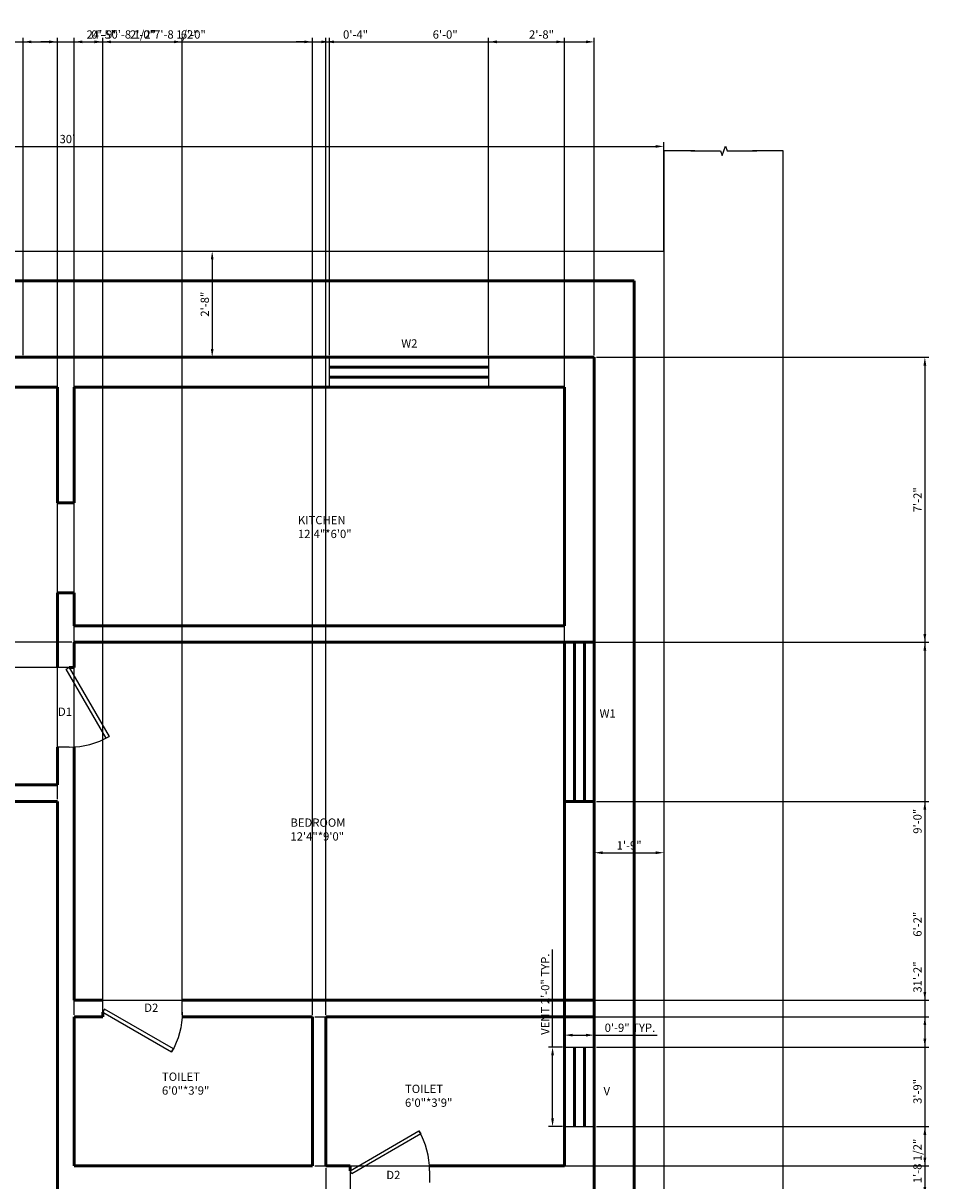
# Model space of a CAD drawing. Units: inches. Extents: x 2020 to 7901, y 1581 to 3943.
# Tile 5 of 17: x 2526 to 2800, y 1966 to 2315. Entities that reach past the tile are written whole.
import ezdxf

# ---------------------------------------------------------------- set-up
doc = ezdxf.new("R2010")
doc.units = ezdxf.units.IN
for name, color, linetype, lineweight in [('A-ANNO-DIMS', 2, 'Continuous', 18), ('A-ANNO-TEXT', 7, 'Continuous', 18), ('A-AREA-IDEN', 3, 'Continuous', 18), ('A-DOOR', 4, 'Continuous', 25), ('A-GLAZ', 4, 'Continuous', 25), ('A-WALL', 7, 'Continuous', 50), ('C-PROP', 6, 'Continuous', 25)]:
    doc.layers.add(name, color=color, linetype=linetype, lineweight=lineweight)
doc.styles.get("Standard").update_dxf_attribs({"font": 'arial.ttf'})
doc.dimstyles.new('ISO-25', dxfattribs={"dimtxt": 2.5, "dimasz": 2.5, "dimexe": 1.25, "dimexo": 0.625, "dimtad": 1, "dimdec": 1, "dimlunit": 3, "dimtxsty": 'Standard', "dimcen": 2.5, "dimadec": 0, "dimazin": 0, "dimtfac": 1, "dimtdec": 1, "dimtmove": 0, "dimatfit": 3, "dimfxl": 1, "dimarcsym": 0})

# ---------------------------------------------------------------- blocks, each defined once
blk = doc.blocks.new('*U2')
for p, q in [((0, 0), (0, -6)), ((40, 0), (40, -6))]:
    blk.add_line(p, q)
blk.add_lwpolyline([(0, 0), (34.64, 20), (35.52, 18.48), (0.87, -1.52)], close=True)
blk.add_arc((0, 0), 40, 0, 30)
blk = doc.blocks.new('*D6')
at = {"layer": 'A-ANNO-DIMS', "color": 0, "lineweight": -2, "transparency": 16777216}
for p, q in [((2574.55, 2246.34), (2583.91, 2246.34)), ((2582.66, 2243.84), (2582.66, 2216.84)), ((2574.55, 2214.34), (2583.91, 2214.34))]:
    blk.add_line(p, q, dxfattribs=at)
at = {"layer": 'A-ANNO-DIMS', "color": 0, "transparency": 16777216}
for points in [[(2582.24, 2243.84), (2583.08, 2243.84), (2582.66, 2246.34)], [(2582.24, 2216.84), (2583.08, 2216.84), (2582.66, 2214.34)]]:
    blk.add_solid(points, dxfattribs=at)
at = {"layer": 'DEFPOINTS', "color": 0, "transparency": 16777216}
for p in [(2573.92, 2246.34), (2573.92, 2214.34), (2582.66, 2214.34)]:
    blk.add_point(p, dxfattribs=at)
at = {"layer": 'A-ANNO-DIMS', "color": 0, "transparency": 16777216, "insert": (2580.76, 2230.34), "char_height": 2.5, "attachment_point": 5, "rotation": 90}
blk.add_mtext('2\'-8"', dxfattribs=at)
blk = doc.blocks.new('*D7')
at = {"layer": 'A-ANNO-DIMS', "color": 0, "lineweight": -2, "transparency": 16777216}
for p, q in [((2697.96, 2068.17), (2697.96, 2063.6)), ((2718.96, 2068.17), (2718.96, 2063.6)), ((2700.46, 2064.85), (2716.46, 2064.85))]:
    blk.add_line(p, q, dxfattribs=at)
at = {"layer": 'A-ANNO-DIMS', "color": 0, "transparency": 16777216}
for points in [[(2700.46, 2065.27), (2700.46, 2064.43), (2697.96, 2064.85)], [(2716.46, 2065.27), (2716.46, 2064.43), (2718.96, 2064.85)]]:
    blk.add_solid(points, dxfattribs=at)
at = {"layer": 'DEFPOINTS', "color": 0, "transparency": 16777216}
for p in [(2697.96, 2068.8), (2718.96, 2068.8), (2718.96, 2064.85)]:
    blk.add_point(p, dxfattribs=at)
at = {"layer": 'A-ANNO-DIMS', "color": 0, "transparency": 16777216, "insert": (2708.46, 2066.75), "char_height": 2.5, "attachment_point": 5}
blk.add_mtext('1\'-9"', dxfattribs=at)
blk = doc.blocks.new('*D8')
at = {"layer": 'A-ANNO-DIMS', "color": 0, "lineweight": -2, "transparency": 16777216}
for p, q in [((2358.96, 2246.96), (2358.96, 2279.19)), ((2361.46, 2277.94), (2716.46, 2277.94)), ((2718.96, 2246.96), (2718.96, 2279.19))]:
    blk.add_line(p, q, dxfattribs=at)
at = {"layer": 'A-ANNO-DIMS', "color": 0, "transparency": 16777216}
for points in [[(2361.46, 2278.35), (2361.46, 2277.52), (2358.96, 2277.94)], [(2716.46, 2278.35), (2716.46, 2277.52), (2718.96, 2277.94)]]:
    blk.add_solid(points, dxfattribs=at)
at = {"layer": 'DEFPOINTS', "color": 0, "transparency": 16777216}
for p in [(2718.96, 2277.94), (2358.96, 2246.34), (2718.96, 2246.34)]:
    blk.add_point(p, dxfattribs=at)
at = {"layer": 'A-ANNO-DIMS', "color": 0, "transparency": 16777216, "insert": (2538.96, 2279.84), "char_height": 2.5, "attachment_point": 5}
blk.add_mtext("30'", dxfattribs=at)
blk = doc.blocks.new('WIN-1200')
for p, q in [((0, 9), (48, 9)), ((0, 0), (0, 9)), ((48, 9), (48, 0)), ((48, 0), (0, 0))]:
    blk.add_line(p, q)
blk = doc.blocks.new('VENT-600')
for p, q in [((0, 24), (9, 24)), ((0, 24), (0, 0)), ((9, 0), (9, 24)), ((0, 0), (9, 0))]:
    blk.add_line(p, q)
blk = doc.blocks.new('*D27')
at = {"layer": 'A-ANNO-DIMS', "color": 0, "lineweight": -2, "transparency": 16777216}
for p, q in [((2685.36, 2006.22), (2685.36, 2035.62)), ((2688.34, 2006.22), (2684.11, 2006.22)), ((2685.36, 1984.72), (2685.36, 2003.72)), ((2688.34, 1982.22), (2684.11, 1982.22))]:
    blk.add_line(p, q, dxfattribs=at)
at = {"layer": 'A-ANNO-DIMS', "color": 0, "transparency": 16777216}
for points in [[(2684.95, 2003.72), (2685.78, 2003.72), (2685.36, 2006.22)], [(2684.95, 1984.72), (2685.78, 1984.72), (2685.36, 1982.22)]]:
    blk.add_solid(points, dxfattribs=at)
at = {"layer": 'DEFPOINTS', "color": 0, "transparency": 16777216}
for p in [(2685.36, 2006.22), (2688.96, 2006.22), (2688.96, 1982.22)]:
    blk.add_point(p, dxfattribs=at)
at = {"layer": 'A-ANNO-DIMS', "color": 0, "transparency": 16777216, "insert": (2683.46, 2022.17), "char_height": 2.5, "attachment_point": 5, "rotation": 90}
blk.add_mtext('VENT 2\'-0" TYP.', dxfattribs=at)
blk = doc.blocks.new('*D28')
at = {"layer": 'A-ANNO-DIMS', "color": 0, "lineweight": -2, "transparency": 16777216}
for p, q in [((2688.96, 2006.84), (2688.96, 2011.07)), ((2691.46, 2009.82), (2695.46, 2009.82)), ((2697.96, 2006.84), (2697.96, 2011.07)), ((2697.96, 2009.82), (2716.95, 2009.82))]:
    blk.add_line(p, q, dxfattribs=at)
at = {"layer": 'A-ANNO-DIMS', "color": 0, "transparency": 16777216}
for points in [[(2691.46, 2010.23), (2691.46, 2009.4), (2688.96, 2009.82)], [(2695.46, 2010.23), (2695.46, 2009.4), (2697.96, 2009.82)]]:
    blk.add_solid(points, dxfattribs=at)
at = {"layer": 'DEFPOINTS', "color": 0, "transparency": 16777216}
for p in [(2697.96, 2009.82), (2688.96, 2006.22), (2697.96, 2006.22)]:
    blk.add_point(p, dxfattribs=at)
at = {"layer": 'A-ANNO-DIMS', "color": 0, "transparency": 16777216, "insert": (2708.71, 2011.72), "char_height": 2.5, "attachment_point": 5}
blk.add_mtext('0\'-9" TYP.', dxfattribs=at)
blk = doc.blocks.new('*D32')
at = {"layer": 'A-ANNO-DIMS', "color": 0, "lineweight": -2, "transparency": 16777216}
for p, q in [((2525.61, 2214.96), (2525.61, 2310.73)), ((2528.11, 2309.48), (2615.57, 2309.48)), ((2618.07, 2214.96), (2618.07, 2310.73))]:
    blk.add_line(p, q, dxfattribs=at)
at = {"layer": 'A-ANNO-DIMS', "color": 0, "transparency": 16777216}
for points in [[(2528.11, 2309.9), (2528.11, 2309.07), (2525.61, 2309.48)], [(2615.57, 2309.9), (2615.57, 2309.07), (2618.07, 2309.48)]]:
    blk.add_solid(points, dxfattribs=at)
at = {"layer": 'DEFPOINTS', "color": 0, "transparency": 16777216}
for p in [(2618.07, 2309.48), (2525.61, 2214.34), (2618.07, 2214.34)]:
    blk.add_point(p, dxfattribs=at)
at = {"layer": 'A-ANNO-DIMS', "color": 0, "transparency": 16777216, "insert": (2571.84, 2311.4), "char_height": 2.5, "attachment_point": 5}
blk.add_mtext('7\'-8 1/2"', dxfattribs=at)
blk = doc.blocks.new('*D33')
at = {"layer": 'A-ANNO-DIMS', "color": 0, "lineweight": -2, "transparency": 16777216}
for p, q in [((2666.07, 2214.96), (2666.07, 2310.73)), ((2668.57, 2309.48), (2695.46, 2309.48)), ((2697.96, 2214.96), (2697.96, 2310.73))]:
    blk.add_line(p, q, dxfattribs=at)
at = {"layer": 'A-ANNO-DIMS', "color": 0, "transparency": 16777216}
for points in [[(2668.57, 2309.9), (2668.57, 2309.07), (2666.07, 2309.48)], [(2695.46, 2309.9), (2695.46, 2309.07), (2697.96, 2309.48)]]:
    blk.add_solid(points, dxfattribs=at)
at = {"layer": 'DEFPOINTS', "color": 0, "transparency": 16777216}
for p in [(2697.96, 2309.48), (2666.07, 2214.34), (2697.96, 2214.34)]:
    blk.add_point(p, dxfattribs=at)
at = {"layer": 'A-ANNO-DIMS', "color": 0, "transparency": 16777216, "insert": (2682.02, 2311.38), "char_height": 2.5, "attachment_point": 5}
blk.add_mtext('2\'-8"', dxfattribs=at)
blk = doc.blocks.new('*D34')
at = {"layer": 'A-ANNO-DIMS', "color": 0, "lineweight": -2, "transparency": 16777216}
for p, q in [((2698.59, 2214.34), (2798.95, 2214.34)), ((2797.7, 2211.84), (2797.7, 2130.84)), ((2698.59, 2128.34), (2798.95, 2128.34))]:
    blk.add_line(p, q, dxfattribs=at)
at = {"layer": 'A-ANNO-DIMS', "color": 0, "transparency": 16777216}
for points in [[(2797.28, 2211.84), (2798.12, 2211.84), (2797.7, 2214.34)], [(2797.28, 2130.84), (2798.12, 2130.84), (2797.7, 2128.34)]]:
    blk.add_solid(points, dxfattribs=at)
at = {"layer": 'DEFPOINTS', "color": 0, "transparency": 16777216}
for p in [(2697.96, 2214.34), (2697.96, 2128.34), (2797.7, 2128.34)]:
    blk.add_point(p, dxfattribs=at)
at = {"layer": 'A-ANNO-DIMS', "color": 0, "transparency": 16777216, "insert": (2795.82, 2171.34), "char_height": 2.5, "attachment_point": 5, "rotation": 90}
blk.add_mtext('7\'-2"', dxfattribs=at)
blk = doc.blocks.new('*D35')
at = {"layer": 'A-ANNO-DIMS', "color": 0, "lineweight": -2, "transparency": 16777216}
for p, q in [((2698.59, 2080.34), (2798.95, 2080.34)), ((2797.7, 2077.84), (2797.7, 2008.72)), ((2698.59, 2006.22), (2798.95, 2006.22))]:
    blk.add_line(p, q, dxfattribs=at)
at = {"layer": 'A-ANNO-DIMS', "color": 0, "transparency": 16777216}
for points in [[(2797.28, 2077.84), (2798.12, 2077.84), (2797.7, 2080.34)], [(2797.28, 2008.72), (2798.12, 2008.72), (2797.7, 2006.22)]]:
    blk.add_solid(points, dxfattribs=at)
at = {"layer": 'DEFPOINTS', "color": 0, "transparency": 16777216}
for p in [(2697.96, 2080.34), (2697.96, 2006.22), (2797.7, 2006.22)]:
    blk.add_point(p, dxfattribs=at)
at = {"layer": 'A-ANNO-DIMS', "color": 0, "transparency": 16777216, "insert": (2795.8, 2043.28), "char_height": 2.5, "attachment_point": 5, "rotation": 90}
blk.add_mtext('6\'-2"', dxfattribs=at)
blk = doc.blocks.new('*D36')
at = {"layer": 'A-ANNO-DIMS', "color": 0, "lineweight": -2, "transparency": 16777216}
for p, q in [((2698.59, 1982.22), (2798.95, 1982.22)), ((2797.7, 1979.72), (2797.7, 1964)), ((2698.59, 1961.5), (2798.95, 1961.5))]:
    blk.add_line(p, q, dxfattribs=at)
at = {"layer": 'A-ANNO-DIMS', "color": 0, "transparency": 16777216}
for points in [[(2797.28, 1979.72), (2798.12, 1979.72), (2797.7, 1982.22)], [(2797.28, 1964), (2798.12, 1964), (2797.7, 1961.5)]]:
    blk.add_solid(points, dxfattribs=at)
at = {"layer": 'DEFPOINTS', "color": 0, "transparency": 16777216}
for p in [(2697.96, 1982.22), (2697.96, 1961.5), (2797.7, 1961.5)]:
    blk.add_point(p, dxfattribs=at)
at = {"layer": 'A-ANNO-DIMS', "color": 0, "transparency": 16777216, "insert": (2795.78, 1971.86), "char_height": 2.5, "attachment_point": 5, "rotation": 90}
blk.add_mtext('1\'-8 1/2"', dxfattribs=at)
blk = doc.blocks.new('*D95')
at = {"layer": 'A-ANNO-DIMS', "color": 0, "lineweight": -2, "transparency": 16777216}
for p, q in [((2400.96, 2214.96), (2400.96, 2310.73)), ((2403.46, 2309.48), (2695.46, 2309.48)), ((2697.96, 2214.96), (2697.96, 2310.73))]:
    blk.add_line(p, q, dxfattribs=at)
at = {"layer": 'A-ANNO-DIMS', "color": 0, "transparency": 16777216}
for points in [[(2403.46, 2309.9), (2403.46, 2309.07), (2400.96, 2309.48)], [(2695.46, 2309.9), (2695.46, 2309.07), (2697.96, 2309.48)]]:
    blk.add_solid(points, dxfattribs=at)
at = {"layer": 'DEFPOINTS', "color": 0, "transparency": 16777216}
for p in [(2697.96, 2309.48), (2400.96, 2214.34), (2697.96, 2214.34)]:
    blk.add_point(p, dxfattribs=at)
at = {"layer": 'A-ANNO-DIMS', "color": 0, "transparency": 16777216, "insert": (2549.46, 2311.38), "char_height": 2.5, "attachment_point": 5}
blk.add_mtext('24\'-9"', dxfattribs=at)
blk = doc.blocks.new('*D96')
at = {"layer": 'A-ANNO-DIMS', "color": 0, "lineweight": -2, "transparency": 16777216}
for p, q in [((2698.59, 2214.34), (2798.95, 2214.34)), ((2797.7, 2211.84), (2797.7, 1842.84)), ((2698.59, 1840.34), (2798.95, 1840.34))]:
    blk.add_line(p, q, dxfattribs=at)
at = {"layer": 'A-ANNO-DIMS', "color": 0, "transparency": 16777216}
for points in [[(2797.28, 2211.84), (2798.12, 2211.84), (2797.7, 2214.34)], [(2797.28, 1842.84), (2798.12, 1842.84), (2797.7, 1840.34)]]:
    blk.add_solid(points, dxfattribs=at)
at = {"layer": 'DEFPOINTS', "color": 0, "transparency": 16777216}
for p in [(2697.96, 2214.34), (2697.96, 1840.34), (2797.7, 1840.34)]:
    blk.add_point(p, dxfattribs=at)
at = {"layer": 'A-ANNO-DIMS', "color": 0, "transparency": 16777216, "insert": (2795.8, 2027.34), "char_height": 2.5, "attachment_point": 5, "rotation": 90}
blk.add_mtext('31\'-2"', dxfattribs=at)
blk = doc.blocks.new('*D99')
at = {"layer": 'A-ANNO-DIMS', "color": 0, "lineweight": -2, "transparency": 16777216}
for p, q in [((2541.59, 2128.34), (2798.95, 2128.34)), ((2797.7, 2125.84), (2797.7, 2022.84)), ((2541.59, 2020.34), (2798.95, 2020.34))]:
    blk.add_line(p, q, dxfattribs=at)
at = {"layer": 'A-ANNO-DIMS', "color": 0, "transparency": 16777216}
for points in [[(2797.28, 2125.84), (2798.12, 2125.84), (2797.7, 2128.34)], [(2797.28, 2022.84), (2798.12, 2022.84), (2797.7, 2020.34)]]:
    blk.add_solid(points, dxfattribs=at)
at = {"layer": 'DEFPOINTS', "color": 0, "transparency": 16777216}
for p in [(2540.96, 2128.34), (2540.96, 2020.34), (2797.7, 2020.34)]:
    blk.add_point(p, dxfattribs=at)
at = {"layer": 'A-ANNO-DIMS', "color": 0, "transparency": 16777216, "insert": (2795.8, 2074.34), "char_height": 2.5, "attachment_point": 5, "rotation": 90}
blk.add_mtext('9\'-0"', dxfattribs=at)
blk = doc.blocks.new('*D100')
at = {"layer": 'A-ANNO-DIMS', "color": 0, "lineweight": -2, "transparency": 16777216}
for p, q in [((2613.59, 2015.34), (2798.95, 2015.34)), ((2797.7, 2012.84), (2797.7, 1972.84)), ((2613.59, 1970.34), (2798.95, 1970.34))]:
    blk.add_line(p, q, dxfattribs=at)
at = {"layer": 'A-ANNO-DIMS', "color": 0, "transparency": 16777216}
for points in [[(2797.28, 2012.84), (2798.12, 2012.84), (2797.7, 2015.34)], [(2797.28, 1972.84), (2798.12, 1972.84), (2797.7, 1970.34)]]:
    blk.add_solid(points, dxfattribs=at)
at = {"layer": 'DEFPOINTS', "color": 0, "transparency": 16777216}
for p in [(2612.96, 2015.34), (2612.96, 1970.34), (2797.7, 1970.34)]:
    blk.add_point(p, dxfattribs=at)
at = {"layer": 'A-ANNO-DIMS', "color": 0, "transparency": 16777216, "insert": (2795.8, 1992.84), "char_height": 2.5, "attachment_point": 5, "rotation": 90}
blk.add_mtext('3\'-9"', dxfattribs=at)
blk = doc.blocks.new('*D102')
at = {"layer": 'A-ANNO-DIMS', "color": 0, "lineweight": -2, "transparency": 16777216}
for p, q in [((2533.46, 2309.48), (2530.96, 2309.48)), ((2535.96, 2080.96), (2535.96, 2310.73)), ((2535.96, 2309.48), (2540.96, 2309.48)), ((2540.96, 2097.4), (2540.96, 2310.73)), ((2543.46, 2309.48), (2553.86, 2309.48))]:
    blk.add_line(p, q, dxfattribs=at)
at = {"layer": 'A-ANNO-DIMS', "color": 0, "transparency": 16777216}
for points in [[(2533.46, 2309.9), (2533.46, 2309.07), (2535.96, 2309.48)], [(2543.46, 2309.9), (2543.46, 2309.07), (2540.96, 2309.48)]]:
    blk.add_solid(points, dxfattribs=at)
at = {"layer": 'DEFPOINTS', "color": 0, "transparency": 16777216}
for p in [(2540.96, 2309.48), (2540.96, 2096.78), (2535.96, 2080.34)]:
    blk.add_point(p, dxfattribs=at)
at = {"layer": 'A-ANNO-DIMS', "color": 0, "transparency": 16777216, "insert": (2549.91, 2311.38), "char_height": 2.5, "attachment_point": 5}
blk.add_mtext('0\'-5"', dxfattribs=at)
blk = doc.blocks.new('*D103')
at = {"layer": 'A-ANNO-DIMS', "color": 0, "lineweight": -2, "transparency": 16777216}
for p, q in [((2540.96, 2015.96), (2540.96, 2310.73)), ((2543.46, 2309.48), (2610.46, 2309.48)), ((2612.96, 2015.96), (2612.96, 2310.73))]:
    blk.add_line(p, q, dxfattribs=at)
at = {"layer": 'A-ANNO-DIMS', "color": 0, "transparency": 16777216}
for points in [[(2543.46, 2309.9), (2543.46, 2309.07), (2540.96, 2309.48)], [(2610.46, 2309.9), (2610.46, 2309.07), (2612.96, 2309.48)]]:
    blk.add_solid(points, dxfattribs=at)
at = {"layer": 'DEFPOINTS', "color": 0, "transparency": 16777216}
for p in [(2612.96, 2309.48), (2540.96, 2015.34), (2612.96, 2015.34)]:
    blk.add_point(p, dxfattribs=at)
at = {"layer": 'A-ANNO-DIMS', "color": 0, "transparency": 16777216, "insert": (2576.96, 2311.38), "char_height": 2.5, "attachment_point": 5}
blk.add_mtext('6\'-0"', dxfattribs=at)
blk = doc.blocks.new('*D104')
at = {"layer": 'A-ANNO-DIMS', "color": 0, "lineweight": -2, "transparency": 16777216}
for p, q in [((2610.46, 2309.48), (2607.96, 2309.48)), ((2612.96, 2015.96), (2612.96, 2310.73)), ((2612.96, 2309.48), (2616.96, 2309.48)), ((2616.96, 2015.96), (2616.96, 2310.73)), ((2619.46, 2309.48), (2629.86, 2309.48))]:
    blk.add_line(p, q, dxfattribs=at)
at = {"layer": 'A-ANNO-DIMS', "color": 0, "transparency": 16777216}
for points in [[(2610.46, 2309.9), (2610.46, 2309.07), (2612.96, 2309.48)], [(2619.46, 2309.9), (2619.46, 2309.07), (2616.96, 2309.48)]]:
    blk.add_solid(points, dxfattribs=at)
at = {"layer": 'DEFPOINTS', "color": 0, "transparency": 16777216}
for p in [(2616.96, 2309.48), (2612.96, 2015.34), (2616.96, 2015.34)]:
    blk.add_point(p, dxfattribs=at)
at = {"layer": 'A-ANNO-DIMS', "color": 0, "transparency": 16777216, "insert": (2625.91, 2311.38), "char_height": 2.5, "attachment_point": 5}
blk.add_mtext('0\'-4"', dxfattribs=at)
blk = doc.blocks.new('*D105')
at = {"layer": 'A-ANNO-DIMS', "color": 0, "lineweight": -2, "transparency": 16777216}
for p, q in [((2616.96, 2015.96), (2616.96, 2310.73)), ((2619.46, 2309.48), (2686.46, 2309.48)), ((2688.96, 2006.84), (2688.96, 2310.73))]:
    blk.add_line(p, q, dxfattribs=at)
at = {"layer": 'A-ANNO-DIMS', "color": 0, "transparency": 16777216}
for points in [[(2619.46, 2309.9), (2619.46, 2309.07), (2616.96, 2309.48)], [(2686.46, 2309.9), (2686.46, 2309.07), (2688.96, 2309.48)]]:
    blk.add_solid(points, dxfattribs=at)
at = {"layer": 'DEFPOINTS', "color": 0, "transparency": 16777216}
for p in [(2688.96, 2309.48), (2616.96, 2015.34), (2688.96, 2006.22)]:
    blk.add_point(p, dxfattribs=at)
at = {"layer": 'A-ANNO-DIMS', "color": 0, "transparency": 16777216, "insert": (2652.96, 2311.38), "char_height": 2.5, "attachment_point": 5}
blk.add_mtext('6\'-0"', dxfattribs=at)
blk = doc.blocks.new('*D107')
at = {"layer": 'A-ANNO-DIMS', "color": 0, "lineweight": -2, "transparency": 16777216}
for p, q in [((2479.8, 2080.96), (2479.8, 2310.73)), ((2482.3, 2309.48), (2533.46, 2309.48)), ((2535.96, 2080.96), (2535.96, 2310.73))]:
    blk.add_line(p, q, dxfattribs=at)
at = {"layer": 'A-ANNO-DIMS', "color": 0, "transparency": 16777216}
for points in [[(2482.3, 2309.9), (2482.3, 2309.07), (2479.8, 2309.48)], [(2533.46, 2309.9), (2533.46, 2309.07), (2535.96, 2309.48)]]:
    blk.add_solid(points, dxfattribs=at)
at = {"layer": 'DEFPOINTS', "color": 0, "transparency": 16777216}
for p in [(2535.96, 2309.48), (2479.8, 2080.34), (2535.96, 2080.34)]:
    blk.add_point(p, dxfattribs=at)
at = {"layer": 'A-ANNO-DIMS', "color": 0, "transparency": 16777216, "insert": (2507.88, 2311.38), "char_height": 2.5, "attachment_point": 5}
blk.add_mtext('4\'-8"', dxfattribs=at)
blk = doc.blocks.new('*D111')
at = {"layer": 'A-ANNO-DIMS', "color": 0, "lineweight": -2, "transparency": 16777216}
for p, q in [((2540.34, 2128.34), (2272.67, 2128.34)), ((2273.92, 2125.84), (2273.92, 2123.23)), ((2540.34, 2120.73), (2272.67, 2120.73)), ((2273.92, 2120.73), (2273.92, 2104.51))]:
    blk.add_line(p, q, dxfattribs=at)
at = {"layer": 'A-ANNO-DIMS', "color": 0, "transparency": 16777216}
for points in [[(2273.5, 2125.84), (2274.33, 2125.84), (2273.92, 2128.34)], [(2273.5, 2123.23), (2274.33, 2123.23), (2273.92, 2120.73)]]:
    blk.add_solid(points, dxfattribs=at)
at = {"layer": 'DEFPOINTS', "color": 0, "transparency": 16777216}
for p in [(2540.96, 2128.34), (2273.92, 2120.73), (2540.96, 2120.73)]:
    blk.add_point(p, dxfattribs=at)
at = {"layer": 'A-ANNO-DIMS', "color": 0, "transparency": 16777216, "insert": (2272, 2111.37), "char_height": 2.5, "attachment_point": 5, "rotation": 90}
blk.add_mtext('0\'-7 1/2"', dxfattribs=at)
blk = doc.blocks.new('*D114')
at = {"layer": 'A-ANNO-DIMS', "color": 0, "lineweight": -2, "transparency": 16777216}
for p, q in [((2540.96, 2020.96), (2540.96, 2310.73)), ((2543.46, 2309.48), (2547.13, 2309.48)), ((2549.63, 2020.96), (2549.63, 2310.73)), ((2549.63, 2309.48), (2565.85, 2309.48))]:
    blk.add_line(p, q, dxfattribs=at)
at = {"layer": 'A-ANNO-DIMS', "color": 0, "transparency": 16777216}
for points in [[(2543.46, 2309.9), (2543.46, 2309.07), (2540.96, 2309.48)], [(2547.13, 2309.9), (2547.13, 2309.07), (2549.63, 2309.48)]]:
    blk.add_solid(points, dxfattribs=at)
at = {"layer": 'DEFPOINTS', "color": 0, "transparency": 16777216}
for p in [(2549.63, 2309.48), (2540.96, 2020.34), (2549.63, 2020.34)]:
    blk.add_point(p, dxfattribs=at)
at = {"layer": 'A-ANNO-DIMS', "color": 0, "transparency": 16777216, "insert": (2558.99, 2311.4), "char_height": 2.5, "attachment_point": 5}
blk.add_mtext('0\'-8 1/2"', dxfattribs=at)
blk = doc.blocks.new('*D115')
at = {"layer": 'A-ANNO-DIMS', "color": 0, "lineweight": -2, "transparency": 16777216}
for p, q in [((2549.63, 2015.96), (2549.63, 2310.73)), ((2552.13, 2309.48), (2571.09, 2309.48)), ((2573.59, 2015.96), (2573.59, 2310.73))]:
    blk.add_line(p, q, dxfattribs=at)
at = {"layer": 'A-ANNO-DIMS', "color": 0, "transparency": 16777216}
for points in [[(2552.13, 2309.9), (2552.13, 2309.07), (2549.63, 2309.48)], [(2571.09, 2309.9), (2571.09, 2309.07), (2573.59, 2309.48)]]:
    blk.add_solid(points, dxfattribs=at)
at = {"layer": 'DEFPOINTS', "color": 0, "transparency": 16777216}
for p in [(2573.59, 2309.48), (2549.63, 2015.34), (2573.59, 2015.34)]:
    blk.add_point(p, dxfattribs=at)
at = {"layer": 'A-ANNO-DIMS', "color": 0, "transparency": 16777216, "insert": (2561.61, 2311.38), "char_height": 2.5, "attachment_point": 5}
blk.add_mtext('2\'-0"', dxfattribs=at)
blk = doc.blocks.new('*D116')
at = {"layer": 'A-ANNO-DIMS', "color": 0, "lineweight": -2, "transparency": 16777216}
for p, q in [((2616.96, 1969.71), (2616.96, 1664.26)), ((2624.26, 1969.71), (2624.26, 1664.26)), ((2619.46, 1665.51), (2621.76, 1665.51)), ((2624.26, 1665.51), (2640.48, 1665.51))]:
    blk.add_line(p, q, dxfattribs=at)
at = {"layer": 'A-ANNO-DIMS', "color": 0, "transparency": 16777216}
for points in [[(2619.46, 1665.92), (2619.46, 1665.09), (2616.96, 1665.51)], [(2621.76, 1665.92), (2621.76, 1665.09), (2624.26, 1665.51)]]:
    blk.add_solid(points, dxfattribs=at)
at = {"layer": 'DEFPOINTS', "color": 0, "transparency": 16777216}
for p in [(2616.96, 1970.34), (2624.26, 1970.34), (2624.26, 1665.51)]:
    blk.add_point(p, dxfattribs=at)
at = {"layer": 'A-ANNO-DIMS', "color": 0, "transparency": 16777216, "insert": (2633.62, 1667.43), "char_height": 2.5, "attachment_point": 5}
blk.add_mtext('0\'-7 1/2"', dxfattribs=at)

msp = doc.modelspace()

# ---------------------------------------------------------------- linework, layer by layer
at = {"layer": 'A-WALL'}
for p, q in [((2367.96, 2237.34), (2709.96, 2237.34)), ((2709.96, 2237.34), (2709.96, 1766.34)), ((2446.34, 2214.34), (2697.96, 2214.34)), ((2618.07, 2211.34), (2666.07, 2211.34)), ((2697.96, 2214.34), (2697.96, 1766.34)), ((2666.07, 2208.34), (2618.07, 2208.34)), ((2446.34, 2205.34), (2535.96, 2205.34)), ((2535.96, 2170.42), (2535.96, 2205.34)), ((2540.96, 2205.34), (2540.96, 2170.42)), ((2540.96, 2205.34), (2688.96, 2205.34)), ((2688.96, 2205.34), (2688.96, 2133.34)), ((2535.96, 2170.42), (2540.96, 2170.42)), ((2535.96, 2143.26), (2540.96, 2143.26)), ((2535.96, 2120.73), (2535.96, 2143.26)), ((2540.96, 2143.26), (2540.96, 2133.34)), ((2540.96, 2133.34), (2688.96, 2133.34)), ((2540.96, 2128.34), (2697.96, 2128.34)), ((2540.96, 2128.34), (2540.96, 2120.73)), ((2688.96, 2080.34), (2688.96, 2128.34)), ((2688.96, 2128.34), (2697.96, 2128.34)), ((2688.96, 2128.34), (2688.96, 1970.34)), ((2691.96, 2080.34), (2691.96, 2128.34)), ((2694.96, 2128.34), (2694.96, 2080.34)), ((2697.96, 2128.34), (2697.96, 2080.34)), ((2539.55, 2120.73), (2540.96, 2120.73)), ((2535.96, 2085.34), (2535.96, 2096.73)), ((2540.96, 2096.78), (2540.96, 2020.34)), ((2479.8, 2085.34), (2535.96, 2085.34)), ((2479.8, 2080.34), (2535.96, 2080.34)), ((2535.96, 1956.67), (2535.96, 2080.34)), ((2697.96, 2080.34), (2688.96, 2080.34)), ((2540.96, 2020.34), (2549.63, 2020.34)), ((2573.63, 2020.34), (2697.96, 2020.34)), ((2540.96, 2015.34), (2549.63, 2015.34)), ((2540.96, 2015.34), (2540.96, 1970.34)), ((2549.63, 2016.74), (2549.63, 2015.34)), ((2573.59, 2015.34), (2612.96, 2015.34)), ((2612.96, 2015.34), (2612.96, 1970.34)), ((2616.96, 2015.34), (2616.96, 1970.34)), ((2616.96, 2015.34), (2697.96, 2015.34)), ((2691.96, 2006.22), (2691.96, 1982.22)), ((2694.96, 1982.22), (2694.96, 2006.22)), ((2540.96, 1970.34), (2612.96, 1970.34)), ((2616.96, 1970.34), (2624.26, 1970.34)), ((2624.26, 1968.92), (2624.26, 1970.34)), ((2648.22, 1970.34), (2688.96, 1970.34))]:
    msp.add_line(p, q, dxfattribs=at)
at = {"layer": 'C-PROP'}
for p, q in [((2718.96, 2276.61), (2718.96, 2246.34)), ((2728.34, 2276.61), (2718.96, 2276.61)), ((2718.96, 2246.34), (2718.96, 2276.61)), ((2718.96, 2246.34), (2718.96, 2276.61)), ((2754.96, 2276.61), (2745.74, 2276.61)), ((2754.96, 1766.34), (2754.96, 2276.61)), ((2358.96, 2246.34), (2718.96, 2246.34)), ((2718.96, 2246.34), (2718.96, 1766.34))]:
    msp.add_line(p, q, dxfattribs=at)
msp.add_lwpolyline([(2727.09, 2276.61), (2736.04, 2276.61), (2736.54, 2275.24), (2737.54, 2277.98), (2738.04, 2276.61), (2746.99, 2276.61)], dxfattribs=at)

# ---------------------------------------------------------------- block references
at = {"layer": 'A-DOOR', "yscale": 0.6, "zscale": 0.6}
for p, xscale, rotation in [((2539.55, 2120.73), 0.6, 270), ((2549.63, 2016.74), -0.6, 180)]:
    msp.add_blockref('*U2', p, dxfattribs=dict(at, xscale=xscale, rotation=rotation))
at = {"layer": 'A-DOOR', "xscale": 0.6, "yscale": 0.6, "zscale": 0.6}
msp.add_blockref('*U2', (2624.26, 1968.92), dxfattribs=at)
at = {"layer": 'A-GLAZ'}
for name, p in [('WIN-1200', (2618.07, 2205.34)), ('VENT-600', (2688.96, 1982.22))]:
    msp.add_blockref(name, p, dxfattribs=at)

# ---------------------------------------------------------------- texts
at = {"layer": 'A-ANNO-TEXT', "char_height": 2.5, "attachment_point": 1}
for s, width, insert in [('W2', 15.2744, (2639.71, 2219.76)), ('D1', 6.5567, (2536.12, 2108.64)), ('W1', 8.0988, (2699.54, 2108.1)), ('D2', 8.3727, (2562.16, 2019.33)), ('V', 8.5448, (2700.75, 1994.16)), ('D2', 8.9578, (2635.2, 1968.88))]:
    msp.add_mtext_dynamic_manual_height_columns(s, width=width, gutter_width=12.5, heights=[0], dxfattribs=dict(at, insert=insert))
at = {"layer": 'A-AREA-IDEN', "char_height": 2.5, "attachment_point": 1}
for s, width, insert in [('KITCHEN\\P12\'4"*6\'0"', 88.2179, (2608.53, 2166.45)), ('BEDROOM\\P12\'4"*9\'0"', 46.1495, (2606.27, 2075.19)), ('TOILET\\P6\'0"*3\'9"', 35.8856, (2567.5, 1998.53)), ('TOILET\\P6\'0"*3\'9"', 33.4398, (2640.84, 1994.86))]:
    msp.add_mtext_dynamic_manual_height_columns(s, width=width, gutter_width=12.5, heights=[0], dxfattribs=dict(at, insert=insert))

# ---------------------------------------------------------------- dimensions: what is measured, and where the dimension line sits
at = {"layer": 'A-ANNO-DIMS'}
for base, p1, p2, override, picture, middle in [((2697.96, 2309.48), (2400.96, 2214.34), (2697.96, 2214.34), {"dimdec": 1, "dimlfac": 1, "dimrnd": 0, "dimzin": 1, "dimdsep": 46, "dimlunit": 4, "dimfrac": 2}, '*D95', (2549.46, 2311.38)), ((2535.96, 2309.48), (2479.8, 2080.34), (2535.96, 2080.34), {"dimdec": 1, "dimlfac": 1, "dimrnd": 0, "dimzin": 1, "dimdsep": 46, "dimlunit": 4, "dimfrac": 2}, '*D107', (2507.88, 2311.38)), ((2618.07, 2309.48), (2525.61, 2214.34), (2618.07, 2214.34), {"dimdec": 1, "dimlfac": 1, "dimrnd": 0, "dimzin": 1, "dimdsep": 46, "dimlunit": 4, "dimfrac": 2}, '*D32', (2571.84, 2311.4)), ((2540.96, 2309.48), (2535.96, 2080.34), (2540.96, 2096.78), {"dimdec": 1, "dimlfac": 1, "dimrnd": 0, "dimzin": 1, "dimdsep": 46, "dimlunit": 4, "dimfrac": 2}, '*D102', (2549.91, 2311.38)), ((2549.63, 2309.48), (2540.96, 2020.34), (2549.63, 2020.34), {"dimdec": 1, "dimlfac": 1, "dimrnd": 0, "dimzin": 1, "dimdsep": 46, "dimlunit": 4, "dimfrac": 2}, '*D114', (2558.99, 2311.4)), ((2612.96, 2309.48), (2540.96, 2015.34), (2612.96, 2015.34), {"dimdec": 1, "dimlfac": 1, "dimrnd": 0, "dimzin": 1, "dimdsep": 46, "dimlunit": 4, "dimfrac": 2}, '*D103', (2576.96, 2311.38)), ((2573.59, 2309.48), (2549.63, 2015.34), (2573.59, 2015.34), {"dimdec": 1, "dimlfac": 1, "dimrnd": 0, "dimzin": 1, "dimdsep": 46, "dimlunit": 4, "dimfrac": 2}, '*D115', (2561.61, 2311.38)), ((2616.96, 2309.48), (2612.96, 2015.34), (2616.96, 2015.34), {"dimdec": 1, "dimlfac": 1, "dimrnd": 0, "dimzin": 1, "dimdsep": 46, "dimlunit": 4, "dimfrac": 2}, '*D104', (2625.91, 2311.38)), ((2688.96, 2309.48), (2616.96, 2015.34), (2688.96, 2006.22), {"dimdec": 1, "dimlfac": 1, "dimrnd": 0, "dimzin": 1, "dimdsep": 46, "dimlunit": 4, "dimfrac": 2}, '*D105', (2652.96, 2311.38)), ((2697.96, 2309.48), (2666.07, 2214.34), (2697.96, 2214.34), {"dimdec": 1, "dimlfac": 1, "dimrnd": 0, "dimzin": 1, "dimdsep": 46, "dimlunit": 4, "dimfrac": 2}, '*D33', (2682.02, 2311.38)), ((2718.96, 2277.94), (2358.96, 2246.34), (2718.96, 2246.34), {"dimclrd": 0, "dimclre": 0, "dimclrt": 0}, '*D8', (2538.96, 2279.84)), ((2718.96, 2064.85), (2697.96, 2068.8), (2718.96, 2068.8), {"dimclrd": 0, "dimclre": 0, "dimclrt": 0}, '*D7', (2708.46, 2066.75)), ((2624.26, 1665.51), (2616.96, 1970.34), (2624.26, 1970.34), {"dimdec": 1, "dimlfac": 1, "dimrnd": 0, "dimzin": 1, "dimdsep": 46, "dimlunit": 4, "dimfrac": 2}, '*D116', (2633.62, 1667.43))]:
    dim = msp.add_linear_dim(base=base, p1=p1, p2=p2, dimstyle='ISO-25', override=override, dxfattribs=at)
    dim.commit()
    dim.dimension.update_dxf_attribs({"geometry": picture, "text_midpoint": middle})
for base, p1, p2, override, picture, middle in [((2582.66, 2214.34), (2573.92, 2246.34), (2573.92, 2214.34), {"dimclrd": 0, "dimclre": 0, "dimclrt": 0}, '*D6', (2580.76, 2230.34)), ((2797.7, 2128.34), (2697.96, 2214.34), (2697.96, 2128.34), {"dimdec": 1, "dimlfac": 1, "dimrnd": 0, "dimzin": 1, "dimdsep": 46, "dimlunit": 4, "dimfrac": 2}, '*D34', (2795.82, 2171.34)), ((2797.7, 1840.34), (2697.96, 2214.34), (2697.96, 1840.34), {"dimdec": 1, "dimlfac": 1, "dimrnd": 0, "dimzin": 1, "dimdsep": 46, "dimlunit": 4, "dimfrac": 2}, '*D96', (2795.8, 2027.34)), ((2273.92, 2120.73), (2540.96, 2128.34), (2540.96, 2120.73), {"dimdec": 1, "dimlfac": 1, "dimrnd": 0, "dimzin": 1, "dimdsep": 46, "dimlunit": 4, "dimfrac": 2}, '*D111', (2272, 2111.37)), ((2797.7, 2020.34), (2540.96, 2128.34), (2540.96, 2020.34), {"dimdec": 1, "dimlfac": 1, "dimrnd": 0, "dimzin": 1, "dimdsep": 46, "dimlunit": 4, "dimfrac": 2}, '*D99', (2795.8, 2074.34)), ((2797.7, 2006.22), (2697.96, 2080.34), (2697.96, 2006.22), {"dimdec": 1, "dimlfac": 1, "dimrnd": 0, "dimzin": 1, "dimdsep": 46, "dimlunit": 4, "dimfrac": 2}, '*D35', (2795.8, 2043.28)), ((2797.7, 1970.34), (2612.96, 2015.34), (2612.96, 1970.34), {"dimdec": 1, "dimlfac": 1, "dimrnd": 0, "dimzin": 1, "dimdsep": 46, "dimlunit": 4, "dimfrac": 2}, '*D100', (2795.8, 1992.84)), ((2797.7, 1961.5), (2697.96, 1982.22), (2697.96, 1961.5), {"dimdec": 1, "dimlfac": 1, "dimrnd": 0, "dimzin": 1, "dimdsep": 46, "dimlunit": 4, "dimfrac": 2}, '*D36', (2795.78, 1971.86))]:
    dim = msp.add_linear_dim(base=base, p1=p1, p2=p2, angle=90, dimstyle='ISO-25', override=override, dxfattribs=at)
    dim.commit()
    dim.dimension.update_dxf_attribs({"geometry": picture, "text_midpoint": middle})
dim = msp.add_linear_dim(base=(2685.36, 2006.22), p1=(2688.96, 1982.22), p2=(2688.96, 2006.22), angle=90, text='VENT <> TYP.', dimstyle='ISO-25', override={"dimdec": 1, "dimrnd": 0, "dimzin": 1, "dimlunit": 4, "dimfrac": 2}, dxfattribs=at)
dim.commit()
dim.dimension.update_dxf_attribs({"geometry": '*D27', "text_midpoint": (2683.46, 2022.17)})
dim = msp.add_linear_dim(base=(2697.96, 2009.82), p1=(2688.96, 2006.22), p2=(2697.96, 2006.22), text='<> TYP.', dimstyle='ISO-25', override={"dimdec": 1, "dimrnd": 0, "dimzin": 1, "dimlunit": 4, "dimfrac": 2}, dxfattribs=at)
dim.commit()
dim.dimension.update_dxf_attribs({"geometry": '*D28', "text_midpoint": (2708.71, 2011.72)})

doc.saveas('drawing.dxf')
